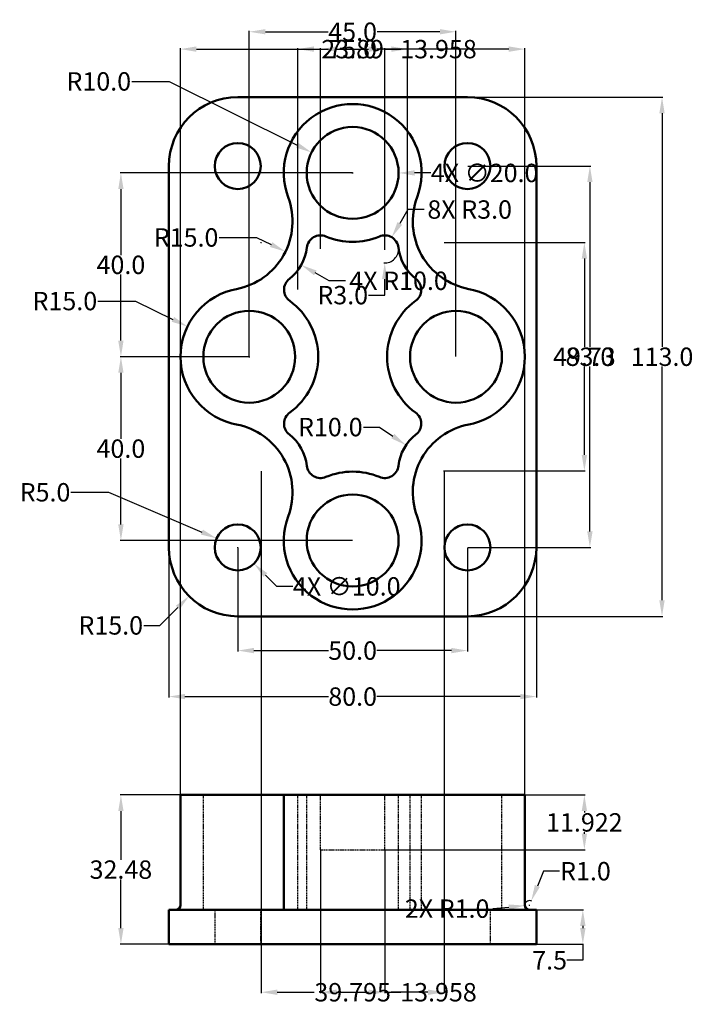
# Model space of a CAD drawing. Units: inches. Extents: x 368 to 514, y 288 to 502.
import ezdxf

# ---------------------------------------------------------------- set-up
doc = ezdxf.new("R2010")
doc.units = ezdxf.units.IN
doc.header["$MEASUREMENT"] = 0
doc.linetypes.add('DASHED2', pattern=[0.375, 0.25, -0.125])
for name, color, linetype, lineweight in [('M-DIMS', 2, 'Continuous', 25), ('M-HIDN', 4, 'DASHED2', 25), ('M-OUTL', 7, 'Continuous', 50)]:
    doc.layers.add(name, color=color, linetype=linetype, lineweight=lineweight)
doc.styles.get("Standard").update_dxf_attribs({"font": 'arial.ttf'})
doc.dimstyles.get("Standard").update_dxf_attribs({"dimtxt": 4, "dimasz": 3.5, "dimexe": 0.18, "dimexo": 0.0625, "dimgap": 0.09, "dimtad": 0, "dimtih": 1, "dimtoh": 1, "dimdec": 1, "dimzin": 0, "dimdsep": 46, "dimtxsty": 'Standard', "dimcen": 0.09, "dimadec": 0, "dimazin": 0, "dimtfac": 1, "dimtdec": 1, "dimtofl": 0, "dimtmove": 0, "dimatfit": 3, "dimfxl": 1, "dimtolj": 1, "dimtzin": 0, "dimarcsym": 0})

# ---------------------------------------------------------------- blocks, each defined once
blk = doc.blocks.new('*D1')
at = {"layer": 'Defpoints', "color": 0, "transparency": 16777216}
for p in [(465.27, 485.34), (465.27, 372.34), (507.62, 372.34)]:
    blk.add_point(p, dxfattribs=at)
at = {"layer": 'M-DIMS', "color": 0, "lineweight": -2, "transparency": 16777216}
for p, q in [((465.33, 485.34), (507.8, 485.34)), ((507.62, 481.84), (507.62, 430.98)), ((507.62, 375.84), (507.62, 426.71)), ((465.33, 372.34), (507.8, 372.34))]:
    blk.add_line(p, q, dxfattribs=at)
at = {"layer": 'M-DIMS', "color": 0, "transparency": 16777216}
for points in [[(507.04, 481.84), (508.2, 481.84), (507.62, 485.34)], [(507.04, 375.84), (508.2, 375.84), (507.62, 372.34)]]:
    blk.add_solid(points, dxfattribs=at)
at = {"layer": 'M-DIMS', "color": 0, "transparency": 16777216, "insert": (507.62, 428.84), "char_height": 4, "attachment_point": 5}
blk.add_mtext('\\A1;113.0', dxfattribs=at)
blk = doc.blocks.new('*D2')
at = {"layer": 'Defpoints', "color": 0, "transparency": 16777216}
for p in [(415.27, 387.34), (465.27, 387.34), (465.27, 364.89)]:
    blk.add_point(p, dxfattribs=at)
at = {"layer": 'M-DIMS', "color": 0, "lineweight": -2, "transparency": 16777216}
for p, q in [((415.27, 387.28), (415.27, 364.71)), ((465.27, 387.28), (465.27, 364.71)), ((418.77, 364.89), (434.99, 364.89)), ((461.77, 364.89), (445.55, 364.89))]:
    blk.add_line(p, q, dxfattribs=at)
at = {"layer": 'M-DIMS', "color": 0, "transparency": 16777216}
for points in [[(418.77, 365.48), (418.77, 364.31), (415.27, 364.89)], [(461.77, 365.48), (461.77, 364.31), (465.27, 364.89)]]:
    blk.add_solid(points, dxfattribs=at)
at = {"layer": 'M-DIMS', "color": 0, "transparency": 16777216, "insert": (440.27, 364.89), "char_height": 4, "attachment_point": 5}
blk.add_mtext('\\A1;50.0', dxfattribs=at)
blk = doc.blocks.new('*D3')
at = {"layer": 'Defpoints', "color": 0, "transparency": 16777216}
for p in [(462.77, 499.57), (417.77, 428.84), (462.77, 428.84)]:
    blk.add_point(p, dxfattribs=at)
at = {"layer": 'M-DIMS', "color": 0, "lineweight": -2, "transparency": 16777216}
for p, q in [((417.77, 428.91), (417.77, 499.75)), ((421.27, 499.57), (434.91, 499.57)), ((459.27, 499.57), (445.63, 499.57)), ((462.77, 428.91), (462.77, 499.75))]:
    blk.add_line(p, q, dxfattribs=at)
at = {"layer": 'M-DIMS', "color": 0, "transparency": 16777216}
for points in [[(421.27, 500.15), (421.27, 498.99), (417.77, 499.57)], [(459.27, 500.15), (459.27, 498.99), (462.77, 499.57)]]:
    blk.add_solid(points, dxfattribs=at)
at = {"layer": 'M-DIMS', "color": 0, "transparency": 16777216, "insert": (440.27, 499.57), "char_height": 4, "attachment_point": 5}
blk.add_mtext('\\A1;45.0', dxfattribs=at)
blk = doc.blocks.new('*D4')
at = {"layer": 'Defpoints', "color": 0, "transparency": 16777216}
for p in [(465.27, 470.34), (465.27, 387.34), (491.92, 387.34)]:
    blk.add_point(p, dxfattribs=at)
at = {"layer": 'M-DIMS', "color": 0, "lineweight": -2, "transparency": 16777216}
for p, q in [((465.33, 470.34), (492.1, 470.34)), ((491.92, 466.84), (491.92, 430.98)), ((491.92, 390.84), (491.92, 426.71)), ((465.33, 387.34), (492.1, 387.34))]:
    blk.add_line(p, q, dxfattribs=at)
at = {"layer": 'M-DIMS', "color": 0, "transparency": 16777216}
for points in [[(491.34, 466.84), (492.51, 466.84), (491.92, 470.34)], [(491.34, 390.84), (492.51, 390.84), (491.92, 387.34)]]:
    blk.add_solid(points, dxfattribs=at)
at = {"layer": 'M-DIMS', "color": 0, "transparency": 16777216, "insert": (491.92, 428.84), "char_height": 4, "attachment_point": 5}
blk.add_mtext('\\A1;83.0', dxfattribs=at)
blk = doc.blocks.new('*D5')
at = {"layer": 'Defpoints', "color": 0, "transparency": 16777216}
for p in [(400.27, 387.34), (480.27, 387.34), (480.27, 354.88)]:
    blk.add_point(p, dxfattribs=at)
at = {"layer": 'M-DIMS', "color": 0, "lineweight": -2, "transparency": 16777216}
for p, q in [((400.27, 387.28), (400.27, 354.7)), ((480.27, 387.28), (480.27, 354.7)), ((403.77, 354.88), (434.99, 354.88)), ((476.77, 354.88), (445.55, 354.88))]:
    blk.add_line(p, q, dxfattribs=at)
at = {"layer": 'M-DIMS', "color": 0, "transparency": 16777216}
for points in [[(403.77, 355.46), (403.77, 354.3), (400.27, 354.88)], [(476.77, 355.46), (476.77, 354.3), (480.27, 354.88)]]:
    blk.add_solid(points, dxfattribs=at)
at = {"layer": 'M-DIMS', "color": 0, "transparency": 16777216, "insert": (440.27, 354.88), "char_height": 4, "attachment_point": 5}
blk.add_mtext('\\A1;80.0', dxfattribs=at)
blk = doc.blocks.new('*D6')
at = {"layer": 'Defpoints', "color": 0, "transparency": 16777216}
for p in [(451.89, 409.59), (460.17, 403.98)]:
    blk.add_point(p, dxfattribs=at)
at = {"layer": 'M-DIMS', "color": 0, "lineweight": -2, "transparency": 16777216}
for p, q in [((442.6, 413.53), (446.1, 413.53)), ((446.1, 413.53), (449, 411.56)), ((460.08, 403.98), (460.26, 403.98)), ((460.17, 403.89), (460.17, 404.07))]:
    blk.add_line(p, q, dxfattribs=at)
at = {"layer": 'M-DIMS', "color": 0, "transparency": 16777216}
blk.add_solid([(449.33, 412.04), (448.67, 411.08), (451.89, 409.59)], dxfattribs=at)
at = {"layer": 'M-DIMS', "color": 0, "transparency": 16777216, "insert": (435.41, 413.53), "char_height": 4, "attachment_point": 5}
blk.add_mtext('\\A1;R10.0', dxfattribs=at)
blk = doc.blocks.new('*D7')
at = {"layer": 'Defpoints', "color": 0, "transparency": 16777216}
for p in [(404.29, 435.43), (417.77, 428.84)]:
    blk.add_point(p, dxfattribs=at)
at = {"layer": 'M-DIMS', "color": 0, "lineweight": -2, "transparency": 16777216}
for p, q in [((384.82, 440.96), (392.98, 440.96)), ((392.98, 440.96), (401.15, 436.97)), ((417.68, 428.84), (417.86, 428.84)), ((417.77, 428.75), (417.77, 428.93))]:
    blk.add_line(p, q, dxfattribs=at)
at = {"layer": 'M-DIMS', "color": 0, "transparency": 16777216}
blk.add_solid([(401.41, 437.49), (400.89, 436.44), (404.29, 435.43)], dxfattribs=at)
at = {"layer": 'M-DIMS', "color": 0, "transparency": 16777216, "insert": (377.62, 440.96), "char_height": 4, "attachment_point": 5}
blk.add_mtext('\\A1;R15.0', dxfattribs=at)
blk = doc.blocks.new('*D8')
at = {"layer": 'Defpoints', "color": 0, "transparency": 16777216}
for p in [(410.67, 389.3), (415.27, 387.34)]:
    blk.add_point(p, dxfattribs=at)
at = {"layer": 'M-DIMS', "color": 0, "lineweight": -2, "transparency": 16777216}
for p, q in [((378.94, 399.34), (387.1, 399.34)), ((387.1, 399.34), (407.45, 390.67)), ((415.18, 387.34), (415.36, 387.34)), ((415.27, 387.25), (415.27, 387.43))]:
    blk.add_line(p, q, dxfattribs=at)
at = {"layer": 'M-DIMS', "color": 0, "transparency": 16777216}
blk.add_solid([(407.68, 391.21), (407.22, 390.14), (410.67, 389.3)], dxfattribs=at)
at = {"layer": 'M-DIMS', "color": 0, "transparency": 16777216, "insert": (373.3, 399.34), "char_height": 4, "attachment_point": 5}
blk.add_mtext('\\A1;R5.0', dxfattribs=at)
blk = doc.blocks.new('*D9')
at = {"layer": 'Defpoints', "color": 0, "transparency": 16777216}
for p in [(431.32, 473.31), (440.27, 468.84)]:
    blk.add_point(p, dxfattribs=at)
at = {"layer": 'M-DIMS', "color": 0, "lineweight": -2, "transparency": 16777216}
for p, q in [((392.19, 488.76), (400.36, 488.76)), ((400.36, 488.76), (428.19, 474.87)), ((440.18, 468.84), (440.36, 468.84)), ((440.27, 468.75), (440.27, 468.93))]:
    blk.add_line(p, q, dxfattribs=at)
at = {"layer": 'M-DIMS', "color": 0, "transparency": 16777216}
blk.add_solid([(428.45, 475.39), (427.93, 474.35), (431.32, 473.31)], dxfattribs=at)
at = {"layer": 'M-DIMS', "color": 0, "transparency": 16777216, "insert": (385, 488.76), "char_height": 4, "attachment_point": 5}
blk.add_mtext('\\A1;R10.0', dxfattribs=at)
blk = doc.blocks.new('*D10')
at = {"layer": 'Defpoints', "color": 0, "transparency": 16777216}
for p in [(447.25, 452.25), (447.25, 449.25)]:
    blk.add_point(p, dxfattribs=at)
at = {"layer": 'M-DIMS', "color": 0, "lineweight": -2, "transparency": 16777216}
for p, q in [((447.16, 452.25), (447.34, 452.25)), ((447.25, 452.16), (447.25, 452.34)), ((447.25, 442.25), (447.25, 445.75)), ((443.75, 442.25), (447.25, 442.25))]:
    blk.add_line(p, q, dxfattribs=at)
blk.add_arc((447.25, 452.25), 3, 266.5623, 5.2372, dxfattribs=at)
at = {"layer": 'M-DIMS', "color": 0, "transparency": 16777216}
blk.add_solid([(446.67, 445.75), (447.83, 445.75), (447.25, 449.25)], dxfattribs=at)
at = {"layer": 'M-DIMS', "color": 0, "transparency": 16777216, "insert": (438.11, 442.25), "char_height": 4, "attachment_point": 5}
blk.add_mtext('\\A1;R3.0', dxfattribs=at)
blk = doc.blocks.new('*D11')
at = {"layer": 'Defpoints', "color": 0, "transparency": 16777216}
for p in [(412.18, 458.32), (425.65, 451.71)]:
    blk.add_point(p, dxfattribs=at)
at = {"layer": 'M-DIMS', "color": 0, "lineweight": -2, "transparency": 16777216}
for p, q in [((411.2, 454.8), (419.36, 454.8)), ((419.36, 454.8), (422.5, 453.25))]:
    blk.add_line(p, q, dxfattribs=at)
at = {"layer": 'M-DIMS', "color": 0, "transparency": 16777216}
blk.add_solid([(422.76, 453.78), (422.25, 452.73), (425.65, 451.71)], dxfattribs=at)
at = {"layer": 'M-DIMS', "color": 0, "transparency": 16777216, "insert": (404.01, 454.8), "char_height": 4, "attachment_point": 5}
blk.add_mtext('\\A1;R15.0', dxfattribs=at)
blk = doc.blocks.new('*D12')
at = {"layer": 'Defpoints', "color": 0, "transparency": 16777216}
for p in [(480.27, 308.48), (480.27, 300.98), (490.38, 300.98)]:
    blk.add_point(p, dxfattribs=at)
at = {"layer": 'M-DIMS', "color": 0, "lineweight": -2, "transparency": 16777216}
for p, q in [((480.33, 308.48), (490.56, 308.48)), ((490.38, 304.98), (490.38, 304.48)), ((480.33, 300.98), (490.56, 300.98)), ((490.38, 300.98), (490.38, 297.48)), ((490.38, 297.48), (486.88, 297.48))]:
    blk.add_line(p, q, dxfattribs=at)
at = {"layer": 'M-DIMS', "color": 0, "transparency": 16777216}
for points in [[(489.8, 304.98), (490.97, 304.98), (490.38, 308.48)], [(489.8, 304.48), (490.97, 304.48), (490.38, 300.98)]]:
    blk.add_solid(points, dxfattribs=at)
at = {"layer": 'M-DIMS', "color": 0, "transparency": 16777216, "insert": (483.15, 297.48), "char_height": 4, "attachment_point": 5}
blk.add_mtext('\\A1;7.5', dxfattribs=at)
blk = doc.blocks.new('*D13')
at = {"layer": 'Defpoints', "color": 0, "transparency": 16777216}
for p in [(478.77, 309.48), (479.15, 310.41)]:
    blk.add_point(p, dxfattribs=at)
at = {"layer": 'M-DIMS', "color": 0, "lineweight": -2, "transparency": 16777216}
for p, q in [((481.81, 316.88), (480.48, 313.64)), ((485.31, 316.88), (481.81, 316.88)), ((478.68, 309.48), (478.86, 309.48)), ((478.77, 309.39), (478.77, 309.57))]:
    blk.add_line(p, q, dxfattribs=at)
blk.add_arc((478.77, 309.48), 1, 57.3768, 176.419, dxfattribs=at)
at = {"layer": 'M-DIMS', "color": 0, "transparency": 16777216}
blk.add_solid([(479.94, 313.87), (481.02, 313.42), (479.15, 310.41)], dxfattribs=at)
at = {"layer": 'M-DIMS', "color": 0, "transparency": 16777216, "insert": (490.95, 316.88), "char_height": 4, "attachment_point": 5}
blk.add_mtext('\\A1;R1.0', dxfattribs=at)
blk = doc.blocks.new('*D14')
at = {"layer": 'Defpoints', "color": 0, "transparency": 16777216}
for p in [(440.27, 468.84), (389.82, 428.84), (417.77, 428.84)]:
    blk.add_point(p, dxfattribs=at)
at = {"layer": 'M-DIMS', "color": 0, "lineweight": -2, "transparency": 16777216}
for p, q in [((440.21, 468.84), (389.64, 468.84)), ((389.82, 465.34), (389.82, 450.97)), ((389.82, 432.34), (389.82, 446.71)), ((417.71, 428.84), (389.64, 428.84))]:
    blk.add_line(p, q, dxfattribs=at)
at = {"layer": 'M-DIMS', "color": 0, "transparency": 16777216}
for points in [[(389.24, 465.34), (390.4, 465.34), (389.82, 468.84)], [(389.24, 432.34), (390.4, 432.34), (389.82, 428.84)]]:
    blk.add_solid(points, dxfattribs=at)
at = {"layer": 'M-DIMS', "color": 0, "transparency": 16777216, "insert": (389.82, 448.84), "char_height": 4, "attachment_point": 5}
blk.add_mtext('\\A1;40.0', dxfattribs=at)
blk = doc.blocks.new('*D15')
at = {"layer": 'Defpoints', "color": 0, "transparency": 16777216}
for p in [(417.77, 428.84), (389.82, 388.84), (440.27, 388.84)]:
    blk.add_point(p, dxfattribs=at)
at = {"layer": 'M-DIMS', "color": 0, "lineweight": -2, "transparency": 16777216}
for p, q in [((417.71, 428.84), (389.64, 428.84)), ((389.82, 425.34), (389.82, 410.97)), ((389.82, 392.34), (389.82, 406.71)), ((440.21, 388.84), (389.64, 388.84))]:
    blk.add_line(p, q, dxfattribs=at)
at = {"layer": 'M-DIMS', "color": 0, "transparency": 16777216}
for points in [[(389.24, 425.34), (390.4, 425.34), (389.82, 428.84)], [(389.24, 392.34), (390.4, 392.34), (389.82, 388.84)]]:
    blk.add_solid(points, dxfattribs=at)
at = {"layer": 'M-DIMS', "color": 0, "transparency": 16777216, "insert": (389.82, 408.84), "char_height": 4, "attachment_point": 5}
blk.add_mtext('\\A1;40.0', dxfattribs=at)
blk = doc.blocks.new('*D16')
at = {"layer": 'Defpoints', "color": 0, "transparency": 16777216}
for p in [(389.82, 333.46), (402.77, 333.46), (400.27, 300.98)]:
    blk.add_point(p, dxfattribs=at)
at = {"layer": 'M-DIMS', "color": 0, "lineweight": -2, "transparency": 16777216}
for p, q in [((402.71, 333.46), (389.64, 333.46)), ((389.82, 329.96), (389.82, 319.36)), ((389.82, 304.48), (389.82, 315.09)), ((400.21, 300.98), (389.64, 300.98))]:
    blk.add_line(p, q, dxfattribs=at)
at = {"layer": 'M-DIMS', "color": 0, "transparency": 16777216}
for points in [[(389.24, 329.96), (390.4, 329.96), (389.82, 333.46)], [(389.24, 304.48), (390.4, 304.48), (389.82, 300.98)]]:
    blk.add_solid(points, dxfattribs=at)
at = {"layer": 'M-DIMS', "color": 0, "transparency": 16777216, "insert": (389.82, 317.22), "char_height": 4, "attachment_point": 5}
blk.add_mtext('\\A1;32.48', dxfattribs=at)
blk = doc.blocks.new('*D17')
at = {"layer": 'Defpoints', "color": 0, "transparency": 16777216}
for p in [(477.77, 495.79), (402.77, 333.46), (477.77, 333.46)]:
    blk.add_point(p, dxfattribs=at)
at = {"layer": 'M-DIMS', "color": 0, "lineweight": -2, "transparency": 16777216}
for p, q in [((402.77, 333.52), (402.77, 495.97)), ((406.27, 495.79), (435.01, 495.79)), ((474.27, 495.79), (445.53, 495.79)), ((477.77, 333.52), (477.77, 495.97))]:
    blk.add_line(p, q, dxfattribs=at)
at = {"layer": 'M-DIMS', "color": 0, "transparency": 16777216}
for points in [[(406.27, 496.38), (406.27, 495.21), (402.77, 495.79)], [(474.27, 496.38), (474.27, 495.21), (477.77, 495.79)]]:
    blk.add_solid(points, dxfattribs=at)
at = {"layer": 'M-DIMS', "color": 0, "transparency": 16777216, "insert": (440.27, 495.79), "char_height": 4, "attachment_point": 5}
blk.add_mtext('\\A1;75.0', dxfattribs=at)
blk = doc.blocks.new('*D18')
at = {"layer": 'Defpoints', "color": 0, "transparency": 16777216}
for p in [(447.25, 333.46), (447.25, 321.54), (490.72, 321.54)]:
    blk.add_point(p, dxfattribs=at)
at = {"layer": 'M-DIMS', "color": 0, "lineweight": -2, "transparency": 16777216}
for p, q in [((447.31, 333.46), (490.9, 333.46)), ((490.72, 329.96), (490.72, 329.63)), ((490.72, 325.04), (490.72, 325.37)), ((447.31, 321.54), (490.9, 321.54))]:
    blk.add_line(p, q, dxfattribs=at)
at = {"layer": 'M-DIMS', "color": 0, "transparency": 16777216}
for points in [[(490.14, 329.96), (491.3, 329.96), (490.72, 333.46)], [(490.14, 325.04), (491.3, 325.04), (490.72, 321.54)]]:
    blk.add_solid(points, dxfattribs=at)
at = {"layer": 'M-DIMS', "color": 0, "transparency": 16777216, "insert": (490.72, 327.5), "char_height": 4, "attachment_point": 5}
blk.add_mtext('\\A1;11.922', dxfattribs=at)
blk = doc.blocks.new('*D19')
at = {"layer": 'Defpoints', "color": 0, "transparency": 16777216}
for p in [(433.29, 321.54), (447.25, 321.54), (447.25, 290.53)]:
    blk.add_point(p, dxfattribs=at)
at = {"layer": 'M-DIMS', "color": 0, "lineweight": -2, "transparency": 16777216}
for p, q in [((433.29, 321.48), (433.29, 290.35)), ((447.25, 321.48), (447.25, 290.35)), ((436.79, 290.53), (443.75, 290.53)), ((447.25, 290.53), (450.75, 290.53))]:
    blk.add_line(p, q, dxfattribs=at)
at = {"layer": 'M-DIMS', "color": 0, "transparency": 16777216}
for points in [[(436.79, 291.12), (436.79, 289.95), (433.29, 290.53)], [(443.75, 291.12), (443.75, 289.95), (447.25, 290.53)]]:
    blk.add_solid(points, dxfattribs=at)
at = {"layer": 'M-DIMS', "color": 0, "transparency": 16777216, "insert": (458.96, 290.53), "char_height": 4, "attachment_point": 5}
blk.add_mtext('\\A1;13.958', dxfattribs=at)
blk = doc.blocks.new('*D20')
at = {"layer": 'Defpoints', "color": 0, "transparency": 16777216}
for p in [(420.37, 403.98), (460.17, 403.98), (460.17, 290.53)]:
    blk.add_point(p, dxfattribs=at)
at = {"layer": 'M-DIMS', "color": 0, "lineweight": -2, "transparency": 16777216}
for p, q in [((420.37, 403.92), (420.37, 290.35)), ((460.17, 403.92), (460.17, 290.35)), ((423.87, 290.53), (431.86, 290.53)), ((456.67, 290.53), (448.68, 290.53))]:
    blk.add_line(p, q, dxfattribs=at)
at = {"layer": 'M-DIMS', "color": 0, "transparency": 16777216}
for points in [[(423.87, 291.12), (423.87, 289.95), (420.37, 290.53)], [(456.67, 291.12), (456.67, 289.95), (460.17, 290.53)]]:
    blk.add_solid(points, dxfattribs=at)
at = {"layer": 'M-DIMS', "color": 0, "transparency": 16777216, "insert": (440.27, 290.53), "char_height": 4, "attachment_point": 5}
blk.add_mtext('\\A1;39.795', dxfattribs=at)
blk = doc.blocks.new('*D21')
at = {"layer": 'Defpoints', "color": 0, "transparency": 16777216}
for p in [(460.17, 453.71), (490.72, 453.71), (460.17, 403.98)]:
    blk.add_point(p, dxfattribs=at)
at = {"layer": 'M-DIMS', "color": 0, "lineweight": -2, "transparency": 16777216}
for p, q in [((460.23, 453.71), (490.9, 453.71)), ((490.72, 450.21), (490.72, 430.98)), ((490.72, 407.48), (490.72, 426.71)), ((460.23, 403.98), (490.9, 403.98))]:
    blk.add_line(p, q, dxfattribs=at)
at = {"layer": 'M-DIMS', "color": 0, "transparency": 16777216}
for points in [[(490.14, 450.21), (491.3, 450.21), (490.72, 453.71)], [(490.14, 407.48), (491.3, 407.48), (490.72, 403.98)]]:
    blk.add_solid(points, dxfattribs=at)
at = {"layer": 'M-DIMS', "color": 0, "transparency": 16777216, "insert": (490.72, 428.84), "char_height": 4, "attachment_point": 5}
blk.add_mtext('\\A1;49.73', dxfattribs=at)
blk = doc.blocks.new('*D22')
at = {"layer": 'Defpoints', "color": 0, "transparency": 16777216}
for p in [(447.25, 495.79), (433.29, 452.25), (447.25, 452.25)]:
    blk.add_point(p, dxfattribs=at)
at = {"layer": 'M-DIMS', "color": 0, "lineweight": -2, "transparency": 16777216}
for p, q in [((433.29, 452.31), (433.29, 495.97)), ((436.79, 495.79), (443.75, 495.79)), ((447.25, 452.31), (447.25, 495.97)), ((447.25, 495.79), (450.75, 495.79))]:
    blk.add_line(p, q, dxfattribs=at)
at = {"layer": 'M-DIMS', "color": 0, "transparency": 16777216}
for points in [[(436.79, 496.38), (436.79, 495.21), (433.29, 495.79)], [(443.75, 496.38), (443.75, 495.21), (447.25, 495.79)]]:
    blk.add_solid(points, dxfattribs=at)
at = {"layer": 'M-DIMS', "color": 0, "transparency": 16777216, "insert": (458.96, 495.79), "char_height": 4, "attachment_point": 5}
blk.add_mtext('\\A1;13.958', dxfattribs=at)
blk = doc.blocks.new('*D23')
at = {"layer": 'Defpoints', "color": 0, "transparency": 16777216}
for p in [(452.22, 495.79), (428.33, 443.42), (452.22, 443.42)]:
    blk.add_point(p, dxfattribs=at)
at = {"layer": 'M-DIMS', "color": 0, "lineweight": -2, "transparency": 16777216}
for p, q in [((428.33, 443.49), (428.33, 495.97)), ((431.83, 495.79), (433.39, 495.79)), ((448.72, 495.79), (447.15, 495.79)), ((452.22, 443.49), (452.22, 495.97))]:
    blk.add_line(p, q, dxfattribs=at)
at = {"layer": 'M-DIMS', "color": 0, "transparency": 16777216}
for points in [[(431.83, 496.38), (431.83, 495.21), (428.33, 495.79)], [(448.72, 496.38), (448.72, 495.21), (452.22, 495.79)]]:
    blk.add_solid(points, dxfattribs=at)
at = {"layer": 'M-DIMS', "color": 0, "transparency": 16777216, "insert": (440.27, 495.79), "char_height": 4, "attachment_point": 5}
blk.add_mtext('\\A1;23.89', dxfattribs=at)
blk = doc.blocks.new('*D24')
at = {"layer": 'Defpoints', "color": 0, "transparency": 16777216}
for p in [(430.27, 468.84), (450.27, 468.84)]:
    blk.add_point(p, dxfattribs=at)
at = {"layer": 'M-DIMS', "color": 0, "lineweight": -2, "transparency": 16777216}
for p, q in [((440.18, 468.84), (440.36, 468.84)), ((440.27, 468.75), (440.27, 468.93)), ((457.27, 468.84), (453.77, 468.84))]:
    blk.add_line(p, q, dxfattribs=at)
at = {"layer": 'M-DIMS', "color": 0, "transparency": 16777216}
blk.add_solid([(453.77, 469.43), (453.77, 468.26), (450.27, 468.84)], dxfattribs=at)
at = {"layer": 'M-DIMS', "color": 0, "transparency": 16777216, "insert": (469, 468.84), "char_height": 4, "attachment_point": 5}
blk.add_mtext('\\A1;4X ∅20.0', dxfattribs=at)
blk = doc.blocks.new('*D25')
at = {"layer": 'Defpoints', "color": 0, "transparency": 16777216}
for p in [(415.27, 387.34), (404.66, 376.74)]:
    blk.add_point(p, dxfattribs=at)
at = {"layer": 'M-DIMS', "color": 0, "lineweight": -2, "transparency": 16777216}
for p, q in [((415.18, 387.34), (415.36, 387.34)), ((415.27, 387.25), (415.27, 387.43)), ((398.3, 370.37), (402.19, 374.26)), ((394.8, 370.37), (398.3, 370.37))]:
    blk.add_line(p, q, dxfattribs=at)
at = {"layer": 'M-DIMS', "color": 0, "transparency": 16777216}
blk.add_solid([(401.78, 374.67), (402.6, 373.85), (404.66, 376.74)], dxfattribs=at)
at = {"layer": 'M-DIMS', "color": 0, "transparency": 16777216, "insert": (387.61, 370.37), "char_height": 4, "attachment_point": 5}
blk.add_mtext('\\A1;R15.0', dxfattribs=at)
blk = doc.blocks.new('*D26')
at = {"layer": 'Defpoints', "color": 0, "transparency": 16777216}
for p in [(411.73, 390.88), (418.81, 383.81)]:
    blk.add_point(p, dxfattribs=at)
at = {"layer": 'M-DIMS', "color": 0, "lineweight": -2, "transparency": 16777216}
for p, q in [((415.18, 387.34), (415.36, 387.34)), ((415.27, 387.25), (415.27, 387.43)), ((423.76, 378.86), (421.28, 381.33)), ((427.26, 378.86), (423.76, 378.86))]:
    blk.add_line(p, q, dxfattribs=at)
at = {"layer": 'M-DIMS', "color": 0, "transparency": 16777216}
blk.add_solid([(421.69, 381.74), (420.87, 380.92), (418.81, 383.81)], dxfattribs=at)
at = {"layer": 'M-DIMS', "color": 0, "transparency": 16777216, "insert": (438.98, 378.86), "char_height": 4, "attachment_point": 5}
blk.add_mtext('\\A1;4X ∅10.0', dxfattribs=at)
blk = doc.blocks.new('*D27')
at = {"layer": 'Defpoints', "color": 0, "transparency": 16777216}
for p in [(420.37, 453.71), (429.09, 448.8)]:
    blk.add_point(p, dxfattribs=at)
at = {"layer": 'M-DIMS', "color": 0, "lineweight": -2, "transparency": 16777216}
for p, q in [((420.28, 453.71), (420.46, 453.71)), ((420.37, 453.62), (420.37, 453.8)), ((435.19, 445.37), (432.14, 447.09)), ((438.69, 445.37), (435.19, 445.37))]:
    blk.add_line(p, q, dxfattribs=at)
at = {"layer": 'M-DIMS', "color": 0, "transparency": 16777216}
blk.add_solid([(432.43, 447.6), (431.85, 446.58), (429.09, 448.8)], dxfattribs=at)
at = {"layer": 'M-DIMS', "color": 0, "transparency": 16777216, "insert": (450.26, 445.37), "char_height": 4, "attachment_point": 5}
blk.add_mtext('\\A1;4X R10.0', dxfattribs=at)
blk = doc.blocks.new('*D28')
at = {"layer": 'Defpoints', "color": 0, "transparency": 16777216}
for p in [(448.77, 454.84), (447.25, 452.25)]:
    blk.add_point(p, dxfattribs=at)
at = {"layer": 'M-DIMS', "color": 0, "lineweight": -2, "transparency": 16777216}
for p, q in [((452.31, 460.88), (450.54, 457.86)), ((455.81, 460.88), (452.31, 460.88)), ((447.16, 452.25), (447.34, 452.25)), ((447.25, 452.16), (447.25, 452.34))]:
    blk.add_line(p, q, dxfattribs=at)
at = {"layer": 'M-DIMS', "color": 0, "transparency": 16777216}
blk.add_solid([(450.03, 458.15), (451.04, 457.56), (448.77, 454.84)], dxfattribs=at)
at = {"layer": 'M-DIMS', "color": 0, "transparency": 16777216, "insert": (465.75, 460.88), "char_height": 4, "attachment_point": 5}
blk.add_mtext('\\A1;8X R3.0', dxfattribs=at)
blk = doc.blocks.new('*D29')
at = {"layer": 'Defpoints', "color": 0, "transparency": 16777216}
for p in [(477.77, 309.39), (478.77, 309.48)]:
    blk.add_point(p, dxfattribs=at)
at = {"layer": 'M-DIMS', "color": 0, "lineweight": -2, "transparency": 16777216}
for p, q in [((470.81, 308.73), (474.29, 309.06)), ((478.68, 309.48), (478.86, 309.48)), ((478.77, 309.39), (478.77, 309.57))]:
    blk.add_line(p, q, dxfattribs=at)
at = {"layer": 'M-DIMS', "color": 0, "transparency": 16777216}
blk.add_solid([(474.24, 309.64), (474.34, 308.48), (477.77, 309.39)], dxfattribs=at)
at = {"layer": 'M-DIMS', "color": 0, "transparency": 16777216, "insert": (460.84, 308.73), "char_height": 4, "attachment_point": 5}
blk.add_mtext('\\A1;2X R1.0', dxfattribs=at)

msp = doc.modelspace()

# ---------------------------------------------------------------- linework, layer by layer
at = {"layer": 'M-HIDN'}
for p, q in [((407.7704, 308.4818), (407.7704, 333.4618)), ((428.3256, 308.4818), (428.3256, 333.4618)), ((430.2704, 308.4818), (430.2704, 333.4618)), ((433.2912, 321.5394), (433.2912, 333.4618)), ((447.2496, 321.5394), (447.2496, 333.4618)), ((450.2704, 308.4818), (450.2704, 333.4618)), ((452.7902, 308.4818), (452.7902, 333.4618)), ((455.2704, 308.4818), (455.2704, 333.4618)), ((472.7704, 308.4818), (472.7704, 333.4618)), ((433.2912, 321.5394), (447.2496, 321.5394)), ((410.2704, 308.4818), (410.2704, 300.9818)), ((420.2704, 300.9818), (420.2704, 308.4818)), ((460.2704, 300.9818), (460.2704, 308.4818)), ((470.2704, 300.9818), (470.2704, 308.4818))]:
    msp.add_line(p, q, dxfattribs=at)
at = {"layer": 'M-OUTL'}
for p, q in [((415.2704, 443.6328), (415.2704, 443.639)), ((465.2704, 443.6328), (465.2704, 443.639)), ((415.2704, 414.0463), (415.2704, 414.0524)), ((465.2704, 414.0463), (465.2704, 414.0524)), ((402.7704, 309.4818), (402.7704, 333.4618)), ((477.7704, 333.4618), (402.7704, 333.4618)), ((425.2704, 308.4818), (425.2704, 333.4618)), ((477.7704, 309.4818), (477.7704, 333.4618)), ((400.2704, 308.4818), (400.2704, 300.9818)), ((480.2704, 308.4818), (400.2704, 308.4818)), ((480.2704, 300.9818), (480.2704, 308.4818)), ((480.2704, 300.9818), (400.2704, 300.9818))]:
    msp.add_line(p, q, dxfattribs=at)
msp.add_lwpolyline([(400.2704, 387.3426, 0.41421356), (415.2704, 372.3426), (465.2704, 372.3426, 0.41421356), (480.2704, 387.3426), (480.2704, 470.3426, 0.41421356), (465.2704, 485.3426), (415.2704, 485.3426, 0.41421356), (400.2704, 470.3426)], format="xyb", close=True, dxfattribs=at)
for centre, radius in [((440.2704, 468.8426), 10), ((415.2704, 470.3426), 5), ((465.2704, 470.3426), 5), ((417.7704, 428.8426), 10), ((462.7704, 428.8426), 10), ((440.2704, 388.8426), 10), ((415.2704, 387.3426), 5), ((465.2704, 387.3426), 5)]:
    msp.add_circle(centre, radius, dxfattribs=at)
for centre, radius, start, end in [((440.2704, 468.8426), 15, 339.459806, 200.540194), ((412.1776, 458.3167), 15, 280.744299, 20.540194), ((468.3632, 458.3167), 15, 159.459806, 259.255701), ((433.2912, 452.2507), 3, 67.186485, 173.569155), ((440.2704, 468.8426), 15, 247.186485, 292.813515), ((447.2496, 452.2507), 3, 6.430845, 112.813515), ((420.373, 453.7068), 10, 307.715338, 353.569155), ((460.1678, 453.7068), 10, 186.430845, 232.284662), ((428.3256, 443.423), 3, 127.715338, 234.098008), ((452.2152, 443.423), 3, 305.901992, 52.284662), ((417.7704, 428.8426), 15, 99.594068, 260.405932), ((462.7704, 428.8426), 15, 279.594068, 80.405932), ((417.7704, 428.8426), 15, 305.901992, 54.098008), ((462.7704, 428.8426), 15, 125.901992, 234.098008), ((428.3256, 414.2623), 3, 125.901992, 232.284662), ((452.2152, 414.2623), 3, 307.715338, 54.098008), ((412.1776, 399.3686), 15, 339.459806, 79.255701), ((468.3632, 399.3686), 15, 100.744299, 200.540194), ((420.373, 403.9785), 10, 6.430845, 52.284662), ((460.1678, 403.9785), 10, 127.715338, 173.569155), ((433.2912, 405.4345), 3, 186.430845, 292.813515), ((447.2496, 405.4345), 3, 247.186485, 353.569155), ((440.2704, 388.8426), 15, 67.186485, 112.813515), ((440.2704, 388.8426), 15, 159.459806, 20.540194), ((401.7704, 309.4818), 1, 270, 0), ((478.7704, 309.4818), 1, 180, 270)]:
    msp.add_arc(centre, radius, start, end, dxfattribs=at)

# ---------------------------------------------------------------- dimensions: what is measured, and where the dimension line sits
at = {"layer": 'M-DIMS'}
for base, p1, p2, override, picture, middle in [((462.7704, 499.5699), (417.7704, 428.8426), (462.7704, 428.8426), {"dimclrd": 0, "dimclre": 0, "dimclrt": 0}, '*D3', (440.2704, 499.5699)), ((477.7704, 495.7926), (402.7704, 333.4618), (477.7704, 333.4618), {"dimdec": 1, "dimlfac": 1, "dimrnd": 0, "dimzin": 0, "dimdsep": 46, "dimlunit": 2}, '*D17', (440.2704, 495.7926)), ((452.2152, 495.7926), (428.3256, 443.423), (452.2152, 443.423), {"dimdec": 2, "dimlfac": 1, "dimrnd": 0, "dimzin": 0, "dimdsep": 46, "dimlunit": 2}, '*D23', (440.2704, 495.7926)), ((447.2496, 495.7926), (433.2912, 452.2507), (447.2496, 452.2507), {"dimdec": 3, "dimlfac": 1, "dimrnd": 0, "dimzin": 0, "dimdsep": 46, "dimlunit": 2}, '*D22', (458.9583, 495.7926)), ((460.1678, 290.5318), (420.373, 403.9785), (460.1678, 403.9785), {"dimdec": 3, "dimlfac": 1, "dimrnd": 0, "dimzin": 0, "dimdsep": 46, "dimlunit": 2}, '*D20', (440.2704, 290.5318)), ((480.2704, 354.8812), (400.2704, 387.3426), (480.2704, 387.3426), {"dimclrd": 0, "dimclre": 0, "dimclrt": 0}, '*D5', (440.2704, 354.8812)), ((465.2704, 364.8923), (415.2704, 387.3426), (465.2704, 387.3426), {"dimclrd": 0, "dimclre": 0, "dimclrt": 0}, '*D2', (440.2704, 364.8923)), ((447.2496, 290.5318), (433.2912, 321.5394), (447.2496, 321.5394), {"dimdec": 3, "dimlfac": 1, "dimrnd": 0, "dimzin": 0, "dimdsep": 46, "dimlunit": 2}, '*D19', (458.9583, 290.5318))]:
    dim = msp.add_linear_dim(base=base, p1=p1, p2=p2, dimstyle='Standard', override=override, dxfattribs=at)
    dim.commit()
    dim.dimension.update_dxf_attribs({"geometry": picture, "text_midpoint": middle})
for center, mpoint, override, picture, middle in [((440.2704, 468.8426), (431.3222, 473.3069), {"dimclrd": 0, "dimclre": 0, "dimclrt": 0}, '*D9', (385.0016, 488.7561)), ((412.1776, 458.3167), (425.646, 451.7135), {"dimclrd": 0, "dimclre": 0, "dimclrt": 0}, '*D11', (404.0068, 454.795)), ((417.7704, 428.8426), (404.2943, 435.4301), {"dimclrd": 0, "dimclre": 0, "dimclrt": 0}, '*D7', (377.6249, 440.9614)), ((415.2704, 387.3426), (410.6703, 389.302), {"dimclrd": 0, "dimclre": 0, "dimclrt": 0}, '*D8', (373.3019, 399.3405)), ((415.2704, 387.3426), (404.6639, 376.7359), {"dimdec": 1, "dimlfac": 1, "dimrnd": 0, "dimzin": 0, "dimdsep": 46, "dimlunit": 2}, '*D25', (387.6077, 370.3719))]:
    dim = msp.add_radius_dim(center=center, mpoint=mpoint, dimstyle='Standard', override=override, dxfattribs=at)
    dim.commit()
    dim.dimension.update_dxf_attribs({"geometry": picture, "text_midpoint": middle, "dimtype": 164})
for base, p1, p2, override, picture, middle in [((507.6195, 372.3426), (465.2704, 485.3426), (465.2704, 372.3426), {"dimclrd": 0, "dimclre": 0, "dimclrt": 0}, '*D1', (507.6195, 428.8426)), ((491.9247, 387.3426), (465.2704, 470.3426), (465.2704, 387.3426), {"dimclrd": 0, "dimclre": 0, "dimclrt": 0}, '*D4', (491.9247, 428.8426)), ((389.8204, 428.8426), (440.2704, 468.8426), (417.7704, 428.8426), {"dimdec": 1, "dimlfac": 1, "dimrnd": 0, "dimzin": 0, "dimdsep": 46, "dimlunit": 2}, '*D14', (389.8204, 448.8426)), ((490.7204, 453.7068), (460.1678, 403.9785), (460.1678, 453.7068), {"dimdec": 2, "dimlfac": 1, "dimrnd": 0, "dimzin": 0, "dimdsep": 46, "dimlunit": 2}, '*D21', (490.7204, 428.8426)), ((389.8204, 388.8426), (417.7704, 428.8426), (440.2704, 388.8426), {"dimdec": 1, "dimlfac": 1, "dimrnd": 0, "dimzin": 0, "dimdsep": 46, "dimlunit": 2}, '*D15', (389.8204, 408.8426)), ((389.8204, 333.4618), (400.2704, 300.9818), (402.7704, 333.4618), {"dimdec": 2, "dimlfac": 1, "dimrnd": 0, "dimzin": 0, "dimdsep": 46, "dimlunit": 2}, '*D16', (389.8204, 317.2218)), ((490.7204, 321.5394), (447.2496, 333.4618), (447.2496, 321.5394), {"dimdec": 3, "dimlfac": 1, "dimrnd": 0, "dimzin": 0, "dimdsep": 46, "dimlunit": 2}, '*D18', (490.7204, 327.5006)), ((490.382, 300.9818), (480.2704, 308.4818), (480.2704, 300.9818), {"dimclrd": 0, "dimclre": 0, "dimclrt": 0}, '*D12', (483.1522, 297.4818))]:
    dim = msp.add_linear_dim(base=base, p1=p1, p2=p2, angle=90, dimstyle='Standard', override=override, dxfattribs=at)
    dim.commit()
    dim.dimension.update_dxf_attribs({"geometry": picture, "text_midpoint": middle})
dim = msp.add_diameter_dim_2p(p1=(430.2704, 468.8423), p2=(450.2704, 468.843), text='4X <>', dimstyle='Standard', override={"dimdec": 1, "dimlfac": 1, "dimrnd": 0, "dimzin": 0, "dimdsep": 46, "dimlunit": 2}, dxfattribs=at)
dim.commit()
dim.dimension.update_dxf_attribs({"geometry": '*D24', "text_midpoint": (457.2704, 468.8433), "dimtype": 163})
for center, mpoint, text, picture, middle in [((447.2496, 452.2507), (448.7669, 454.8388), '8X <>', '*D28', (465.7457, 460.8775)), ((420.373, 453.7068), (429.0887, 448.8041), '4X <>', '*D27', (450.26, 445.3723)), ((478.7704, 309.4818), (477.7748, 309.3882), '2X <>', '*D29', (460.8355, 308.7333))]:
    dim = msp.add_radius_dim(center=center, mpoint=mpoint, text=text, dimstyle='Standard', override={"dimdec": 1, "dimlfac": 1, "dimrnd": 0, "dimzin": 0, "dimdsep": 46, "dimlunit": 2}, dxfattribs=at)
    dim.commit()
    dim.dimension.update_dxf_attribs({"geometry": picture, "text_midpoint": middle})
for center, mpoint, picture, middle in [((447.2496, 452.2507), (447.2496, 449.2507), '*D10', (438.1112, 442.2507)), ((460.1678, 403.9785), (451.8938, 409.5946), '*D6', (435.4097, 413.5259)), ((478.7704, 309.4818), (479.15, 310.4069), '*D13', (490.9458, 316.883))]:
    dim = msp.add_radius_dim(center=center, mpoint=mpoint, dimstyle='Standard', override={"dimclrd": 0, "dimclre": 0, "dimclrt": 0}, dxfattribs=at)
    dim.commit()
    dim.dimension.update_dxf_attribs({"geometry": picture, "text_midpoint": middle})
dim = msp.add_diameter_dim_2p(p1=(411.7349, 390.8782), p2=(418.8059, 383.8071), text='4X <>', dimstyle='Standard', override={"dimdec": 1, "dimlfac": 1, "dimrnd": 0, "dimzin": 0, "dimdsep": 46, "dimlunit": 2}, dxfattribs=at)
dim.commit()
dim.dimension.update_dxf_attribs({"geometry": '*D26', "text_midpoint": (438.9814, 378.8573)})

doc.saveas('drawing.dxf')
